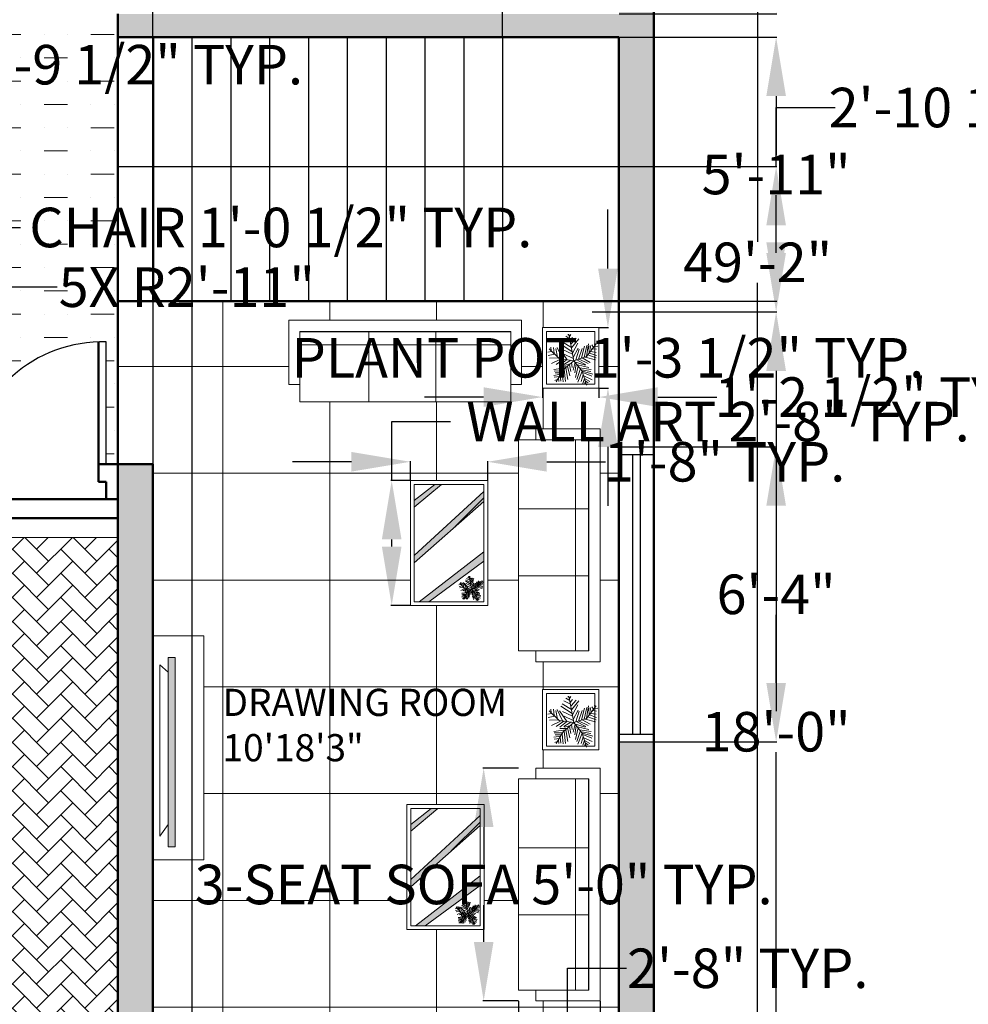
# Model space of a CAD drawing. Units: inches. Extents: x 26 to 14419, y 2 to 3479.
# Tile 3 of 9: x 13759 to 14003, y 2946 to 3199. Entities that reach past the tile are written whole.
import ezdxf

# ---------------------------------------------------------------- set-up
doc = ezdxf.new("R2010")
doc.units = ezdxf.units.IN
doc.header["$MEASUREMENT"] = 0
for name, color, linetype, lineweight in [('A-ANNO-DIMS', 2, 'Continuous', 18), ('A-AREA-IDEN', 7, 'Continuous', 18), ('A-DOOR', 4, 'Continuous', 25), ('A-FLOR-PATT', 252, 'Continuous', 13), ('A-FLOR-STRS', 2, 'Continuous', 25), ('A-FURN', 8, 'Continuous', 18), ('A-GLAZ', 3, 'Continuous', 25), ('A-WALL', 7, 'Continuous', 50), ('L-PLNT', 3, 'Continuous', 13)]:
    doc.layers.add(name, color=color, linetype=linetype, lineweight=lineweight)
doc.styles.get("Standard").update_dxf_attribs({"font": 'arial.ttf'})
doc.dimstyles.get("Standard").update_dxf_attribs({"dimtxt": 10.18, "dimasz": 15.18, "dimexe": 0.18, "dimexo": 0.0625, "dimgap": 0.09, "dimtad": 0, "dimtih": 1, "dimtoh": 1, "dimdec": 0, "dimzin": 0, "dimdsep": 46, "dimlunit": 3, "dimtxsty": 'Standard', "dimcen": 0.09, "dimadec": 0, "dimazin": 0, "dimtfac": 1, "dimtdec": 0, "dimtofl": 0, "dimtmove": 0, "dimatfit": 3, "dimfxl": 1, "dimtolj": 1, "dimtzin": 0, "dimarcsym": 0})

# ---------------------------------------------------------------- blocks, each defined once
blk = doc.blocks.new('*U5')
for p, q in [((-7.288, 39.707), (-21.778, 46.673)), ((-8.737, 47.138), (-17.069, 52.711)), ((-10.186, 53.64), (-13.084, 55.962)), ((0, 0), (-10.5, 57)), ((-9.099, 51.782), (-6.563, 55.962)), ((-7.65, 43.423), (-2.578, 49.46)), ((-5.839, 35.992), (4.667, 48.067)), ((-5.114, 27.632), (10.463, 46.673)), ((-31.5, 4.5), (-52.5, 25.5)), ((-48.585, 21.131), (-49.309, 29.026)), ((-43.513, 28.561), (-42.427, 15.558)), ((-38.442, 26.239), (-34.819, 7.663)), ((-35.544, 28.097), (-24.314, 3.947)), ((-14.533, 2.09), (-30.834, 25.31)), ((-3.665, 19.273), (-27.574, 35.527)), ((-5.114, 28.097), (-24.676, 40.636)), ((-24.314, 23.917), (-2.941, 13.7)), ((-2.941, 16.486), (8.652, 37.85)), ((-1.129, 6.734), (9.014, 26.704)), ((3.942, 1.625), (11.187, 24.381)), ((10.101, 3.483), (17.708, 26.239)), ((16.259, 5.805), (23.142, 31.348)), ((22.055, 7.198), (27.489, 32.277)), ((27, 9), (48, 36)), ((27.127, 9.056), (31.112, 35.992)), ((31.836, 30.883), (32.561, 16.486)), ((35.096, 32.741), (37.27, 22.524)), ((38.719, 34.134), (41.979, 28.561)), ((40.53, 25.775), (48.862, 24.846)), ((43.791, 29.954), (51.036, 30.883)), ((44.153, 36.456), (45.239, 32.741)), ((-47.498, 19.737), (-55.83, 18.344)), ((-40.615, 13.7), (-55.105, 10.913)), ((-33.37, 6.269), (-52.207, 5.34)), ((-28.299, 3.483), (-47.86, -5.805)), ((-21.416, 3.018), (-38.079, -8.128)), ((0, 0), (-31.5, 4.5)), ((-15.982, 2.09), (-30.11, -9.521)), ((0, 0), (-22.5, -19.5)), ((-6.563, 1.161), (-21.416, -8.128)), ((-20.691, 13.7), (-1.129, 4.876)), ((0, 0), (27, 9)), ((0, 0), (18, -22.5)), ((6.478, 1.625), (26.04, -8.592)), ((11.187, 3.483), (30.749, -5.805)), ((18.07, 5.805), (35.096, -3.483)), ((24.229, 7.663), (46.688, 1.625)), ((29.662, 12.307), (48.137, 6.269)), ((33.285, 16.486), (48.862, 10.913)), ((36.183, 19.737), (48.137, 17.88)), ((-17.431, -15.094), (-42.789, -18.809)), ((-22.5, -19.5), (-37.5, -45)), ((-15.257, -12.772), (-30.11, -12.772)), ((-20.691, -18.345), (-17.793, -44.352)), ((-6.563, -5.805), (-19.967, -9.985)), ((-17.069, -15.094), (-12.721, -40.172)), ((-13.446, -11.378), (-8.737, -32.741)), ((-9.461, -8.592), (-6.201, -23.453)), ((-4.752, -3.483), (-3.665, -14.629)), ((2.493, -3.019), (-1.491, -20.202)), ((1.769, -2.555), (24.229, -9.521)), ((5.029, -6.27), (2.131, -25.775)), ((9.014, -11.378), (3.58, -35.992)), ((14.085, -16.951), (6.478, -40.172)), ((7.565, -9.056), (32.198, -14.629)), ((12.274, -15.094), (36.907, -18.809)), ((16.259, -19.738), (36.183, -22.989)), ((-28.299, -29.026), (-42.789, -31.348)), ((-24.314, -21.596), (-42.427, -22.06)), ((-30.834, -34.135), (-42.427, -35.528)), ((-34.457, -39.708), (-40.978, -42.494)), ((-26.849, -26.24), (-40.253, -25.775)), ((-32.646, -36.921), (-31.921, -44.352)), ((-29.023, -30.884), (-27.936, -43.887)), ((-25.038, -23.918), (-22.865, -45.281)), ((18.07, -22.524), (8.289, -45.745)), ((20.244, -30.419), (15.897, -44.816)), ((18, -22.5), (27, -52.5)), ((18.433, -22.524), (40.53, -29.026)), ((19.157, -25.311), (38.719, -33.206)), ((22.78, -37.85), (19.519, -48.532)), ((21.331, -32.741), (39.081, -40.636)), ((22.78, -38.314), (34.372, -44.816)), ((24.591, -45.745), (23.142, -50.854)), ((24.591, -43.423), (30.749, -47.603)), ((26.764, -49.925), (28.213, -50.854))]:
    blk.add_line(p, q)
blk = doc.blocks.new('*D7')
at = {"layer": 'A-ANNO-DIMS', "color": 0, "lineweight": -2, "transparency": 16777216}
for p, q in [((13922.15, 3432), (13949, 3432)), ((13948.82, 3416.82), (13948.82, 3142.28)), ((13948.82, 2857.18), (13948.82, 3131.71)), ((13922.15, 2842), (13949, 2842))]:
    blk.add_line(p, q, dxfattribs=at)
at = {"layer": 'A-ANNO-DIMS', "color": 0, "transparency": 16777216}
for points in [[(13946.29, 3416.82), (13951.35, 3416.82), (13948.82, 3432)], [(13946.29, 2857.18), (13951.35, 2857.18), (13948.82, 2842)]]:
    blk.add_solid(points, dxfattribs=at)
at = {"layer": 'Defpoints', "color": 0, "transparency": 16777216}
for p in [(13922.09, 3432), (13922.09, 2842), (13948.82, 2842)]:
    blk.add_point(p, dxfattribs=at)
at = {"layer": 'A-ANNO-DIMS', "color": 0, "transparency": 16777216, "insert": (13948.82, 3137), "char_height": 10.18, "attachment_point": 5}
blk.add_mtext('\\A1;49\'-2"', dxfattribs=at)
blk = doc.blocks.new('SOFA-3SEAT')
for points in [[(2.79, 18.06), (2.79, 4.46), (0, 4.46), (0, 20.99), (2.79, 20.99)], [(2.79, 20.99), (59.95, 20.99)], [(57.16, 20.99), (59.95, 20.99), (59.95, 4.46), (57.16, 4.46), (57.16, 18.06)], [(57.16, 18.06), (2.79, 18.06)]]:
    blk.add_lwpolyline(points)
blk.add_lwpolyline([(2.79, 18.02), (57.16, 18.02), (57.16, 0), (2.79, 0)], close=True)
blk = doc.blocks.new('DOOR-DOUBLE')
for p, q in [((0, 0), (0, 31.5)), ((72, 0), (72, 31.5)), ((36.16, 0), (35.84, 0))]:
    blk.add_line(p, q)
for centre, start, end in [((1, -3.5), 5.7368, 91.6366), ((71, -3.5), 88.3634, 174.2632)]:
    blk.add_arc(centre, 35.01, start, end)
blk = doc.blocks.new('WALL-ART')
for p, q in [((6.28, 31.2), (1, 27.1)), ((8.01, 31.2), (1, 25.34)), ((18.91, 29.38), (1, 12.87)), ((18.91, 26.84), (1, 10.99)), ((18.91, 13.81), (2.23, 1)), ((18.91, 11.4), (4.72, 1))]:
    blk.add_line(p, q)
for points in [[(0, 32.2), (19.91, 32.2), (19.91, 0), (0, 0)], [(1, 31.2), (18.91, 31.2), (18.91, 1), (1, 1)]]:
    blk.add_lwpolyline(points, close=True)
blk = doc.blocks.new('PLANT-POT')
for points in [[(0, 15.58), (14.52, 15.58), (14.52, 0), (0, 0)], [(1, 14.58), (13.52, 14.58), (13.52, 1), (1, 1)]]:
    blk.add_lwpolyline(points, close=True)
blk = doc.blocks.new('*D23')
at = {"layer": 'A-ANNO-DIMS', "color": 0, "lineweight": -2, "transparency": 16777216}
for p, q in [((13716.08, 3147.8), (13716.08, 3145.8)), ((13728.65, 3147.8), (13728.65, 3145.8)), ((13700.9, 3145.98), (13685.72, 3145.98)), ((13743.83, 3145.98), (13759.01, 3145.98))]:
    blk.add_line(p, q, dxfattribs=at)
at = {"layer": 'A-ANNO-DIMS', "color": 0, "transparency": 16777216}
for points in [[(13700.9, 3148.51), (13700.9, 3143.45), (13716.08, 3145.98)], [(13743.83, 3148.51), (13743.83, 3143.45), (13728.65, 3145.98)]]:
    blk.add_solid(points, dxfattribs=at)
at = {"layer": 'Defpoints', "color": 0, "transparency": 16777216}
for p in [(13716.08, 3147.87), (13728.65, 3147.87), (13728.65, 3145.98)]:
    blk.add_point(p, dxfattribs=at)
at = {"layer": 'A-ANNO-DIMS', "color": 0, "transparency": 16777216, "insert": (13826.02, 3145.98), "char_height": 10.18, "attachment_point": 5}
blk.add_mtext('\\A1;CHAIR 1\'-0 1/2" TYP.', dxfattribs=at)
blk = doc.blocks.new('*D24')
at = {"layer": 'A-ANNO-DIMS', "color": 0, "lineweight": -2, "transparency": 16777216}
for p, q in [((13730.53, 3172.73), (13730.53, 3187.91)), ((13730.53, 3187.91), (13745.71, 3187.91)), ((13728.71, 3157.55), (13730.71, 3157.55)), ((13728.71, 3147.87), (13730.71, 3147.87)), ((13730.53, 3132.69), (13730.53, 3117.51))]:
    blk.add_line(p, q, dxfattribs=at)
at = {"layer": 'A-ANNO-DIMS', "color": 0, "transparency": 16777216}
for points in [[(13728, 3172.73), (13733.06, 3172.73), (13730.53, 3157.55)], [(13728, 3132.69), (13733.06, 3132.69), (13730.53, 3147.87)]]:
    blk.add_solid(points, dxfattribs=at)
at = {"layer": 'Defpoints', "color": 0, "transparency": 16777216}
for p in [(13728.65, 3157.55), (13730.53, 3157.55), (13728.65, 3147.87)]:
    blk.add_point(p, dxfattribs=at)
at = {"layer": 'A-ANNO-DIMS', "color": 0, "transparency": 16777216, "insert": (13788.69, 3187.91), "char_height": 10.18, "attachment_point": 5}
blk.add_mtext('\\A1;0\'-9 1/2" TYP.', dxfattribs=at)
blk = doc.blocks.new('*D30')
at = {"layer": 'A-ANNO-DIMS', "color": 0, "lineweight": -2, "transparency": 16777216}
for p, q in [((13899.89, 2940.02), (13899.89, 2955.2)), ((13899.89, 2955.2), (13915.07, 2955.2)), ((13889.15, 2940.02), (13900.07, 2940.02)), ((13899.89, 2923.18), (13899.89, 2924.84)), ((13889.15, 2908), (13900.07, 2908))]:
    blk.add_line(p, q, dxfattribs=at)
at = {"layer": 'A-ANNO-DIMS', "color": 0, "transparency": 16777216}
for points in [[(13897.36, 2924.84), (13902.42, 2924.84), (13899.89, 2940.02)], [(13897.36, 2923.18), (13902.42, 2923.18), (13899.89, 2908)]]:
    blk.add_solid(points, dxfattribs=at)
at = {"layer": 'Defpoints', "color": 0, "transparency": 16777216}
for p in [(13889.09, 2940.02), (13899.89, 2940.02), (13889.09, 2908)]:
    blk.add_point(p, dxfattribs=at)
at = {"layer": 'A-ANNO-DIMS', "color": 0, "transparency": 16777216, "insert": (13946.27, 2955.2), "char_height": 10.18, "attachment_point": 5}
blk.add_mtext('\\A1;2\'-8" TYP.', dxfattribs=at)
blk = doc.blocks.new('*D31')
at = {"layer": 'A-ANNO-DIMS', "color": 0, "lineweight": -2, "transparency": 16777216}
for p, q in [((13887.2, 3006.75), (13878.09, 3006.75)), ((13878.27, 2991.57), (13878.27, 2982.14)), ((13878.27, 2961.99), (13878.27, 2971.42)), ((13887.2, 2946.81), (13878.09, 2946.81))]:
    blk.add_line(p, q, dxfattribs=at)
at = {"layer": 'A-ANNO-DIMS', "color": 0, "transparency": 16777216}
for points in [[(13875.74, 2991.57), (13880.8, 2991.57), (13878.27, 3006.75)], [(13875.74, 2961.99), (13880.8, 2961.99), (13878.27, 2946.81)]]:
    blk.add_solid(points, dxfattribs=at)
at = {"layer": 'Defpoints', "color": 0, "transparency": 16777216}
for p in [(13887.26, 3006.75), (13878.27, 2946.81), (13887.26, 2946.81)]:
    blk.add_point(p, dxfattribs=at)
at = {"layer": 'A-ANNO-DIMS', "color": 0, "transparency": 16777216, "insert": (13878.27, 2976.78), "char_height": 10.18, "attachment_point": 5}
blk.add_mtext('\\A1;3-SEAT SOFA 5\'-0" TYP.', dxfattribs=at)
blk = doc.blocks.new('*D32')
at = {"layer": 'A-ANNO-DIMS', "color": 0, "lineweight": -2, "transparency": 16777216}
for p, q in [((13887.26, 2946.75), (13887.26, 2937.64)), ((13908.25, 2946.75), (13908.25, 2937.64)), ((13872.08, 2937.82), (13856.9, 2937.82)), ((13923.43, 2937.82), (13938.61, 2937.82))]:
    blk.add_line(p, q, dxfattribs=at)
at = {"layer": 'A-ANNO-DIMS', "color": 0, "transparency": 16777216}
for points in [[(13872.08, 2940.35), (13872.08, 2935.29), (13887.26, 2937.82)], [(13923.43, 2940.35), (13923.43, 2935.29), (13908.25, 2937.82)]]:
    blk.add_solid(points, dxfattribs=at)
at = {"layer": 'Defpoints', "color": 0, "transparency": 16777216}
for p in [(13887.26, 2946.81), (13908.25, 2946.81), (13908.25, 2937.82)]:
    blk.add_point(p, dxfattribs=at)
at = {"layer": 'A-ANNO-DIMS', "color": 0, "transparency": 16777216, "insert": (13969.25, 2937.82), "char_height": 10.18, "attachment_point": 5}
blk.add_mtext('\\A1;1\'-9" TYP.', dxfattribs=at)
blk = doc.blocks.new('*D41')
at = {"layer": 'A-ANNO-DIMS', "color": 0, "lineweight": -2, "transparency": 16777216}
for p, q in [((13854.58, 3080.81), (13854.58, 3095.99)), ((13854.58, 3095.99), (13869.76, 3095.99)), ((13859.35, 3080.81), (13854.4, 3080.81)), ((13854.58, 3063.79), (13854.58, 3065.63)), ((13859.35, 3048.61), (13854.4, 3048.61))]:
    blk.add_line(p, q, dxfattribs=at)
at = {"layer": 'A-ANNO-DIMS', "color": 0, "transparency": 16777216}
for points in [[(13852.05, 3065.63), (13857.11, 3065.63), (13854.58, 3080.81)], [(13852.05, 3063.79), (13857.11, 3063.79), (13854.58, 3048.61)]]:
    blk.add_solid(points, dxfattribs=at)
at = {"layer": 'Defpoints', "color": 0, "transparency": 16777216}
for p in [(13854.58, 3080.81), (13859.41, 3080.81), (13859.41, 3048.61)]:
    blk.add_point(p, dxfattribs=at)
at = {"layer": 'A-ANNO-DIMS', "color": 0, "transparency": 16777216, "insert": (13938.62, 3095.99), "char_height": 10.18, "attachment_point": 5}
blk.add_mtext('\\A1;WALL ART 2\'-8" TYP.', dxfattribs=at)
blk = doc.blocks.new('*D42')
at = {"layer": 'A-ANNO-DIMS', "color": 0, "lineweight": -2, "transparency": 16777216}
for p, q in [((13844.23, 3085.64), (13829.05, 3085.64)), ((13859.41, 3080.87), (13859.41, 3085.82)), ((13879.32, 3080.87), (13879.32, 3085.82)), ((13894.5, 3085.64), (13909.68, 3085.64))]:
    blk.add_line(p, q, dxfattribs=at)
at = {"layer": 'A-ANNO-DIMS', "color": 0, "transparency": 16777216}
for points in [[(13844.23, 3088.17), (13844.23, 3083.11), (13859.41, 3085.64)], [(13894.5, 3088.17), (13894.5, 3083.11), (13879.32, 3085.64)]]:
    blk.add_solid(points, dxfattribs=at)
at = {"layer": 'Defpoints', "color": 0, "transparency": 16777216}
for p in [(13879.32, 3085.64), (13859.41, 3080.81), (13879.32, 3080.81)]:
    blk.add_point(p, dxfattribs=at)
at = {"layer": 'A-ANNO-DIMS', "color": 0, "transparency": 16777216, "insert": (13940.31, 3085.64), "char_height": 10.18, "attachment_point": 5}
blk.add_mtext('\\A1;1\'-8" TYP.', dxfattribs=at)
blk = doc.blocks.new('*D45')
at = {"layer": 'A-ANNO-DIMS', "color": 0, "lineweight": -2, "transparency": 16777216}
for p, q in [((13910.27, 3135.39), (13910.27, 3150.57)), ((13907.99, 3120.21), (13910.45, 3120.21)), ((13907.99, 3104.63), (13910.45, 3104.63)), ((13910.27, 3089.45), (13910.27, 3074.27))]:
    blk.add_line(p, q, dxfattribs=at)
at = {"layer": 'A-ANNO-DIMS', "color": 0, "transparency": 16777216}
for points in [[(13907.74, 3135.39), (13912.8, 3135.39), (13910.27, 3120.21)], [(13907.74, 3089.45), (13912.8, 3089.45), (13910.27, 3104.63)]]:
    blk.add_solid(points, dxfattribs=at)
at = {"layer": 'Defpoints', "color": 0, "transparency": 16777216}
for p in [(13907.93, 3120.21), (13910.27, 3120.21), (13907.93, 3104.63)]:
    blk.add_point(p, dxfattribs=at)
at = {"layer": 'A-ANNO-DIMS', "color": 0, "transparency": 16777216, "insert": (13910.27, 3112.42), "char_height": 10.18, "attachment_point": 5}
blk.add_mtext('\\A1;PLANT POT 1\'-3 1/2" TYP.', dxfattribs=at)
blk = doc.blocks.new('*D46')
at = {"layer": 'A-ANNO-DIMS', "color": 0, "lineweight": -2, "transparency": 16777216}
for p, q in [((13893.41, 3104.57), (13893.41, 3102.12)), ((13907.93, 3104.57), (13907.93, 3102.12)), ((13878.23, 3102.3), (13863.05, 3102.3)), ((13923.11, 3102.3), (13938.29, 3102.3))]:
    blk.add_line(p, q, dxfattribs=at)
at = {"layer": 'A-ANNO-DIMS', "color": 0, "transparency": 16777216}
for points in [[(13878.23, 3104.83), (13878.23, 3099.77), (13893.41, 3102.3)], [(13923.11, 3104.83), (13923.11, 3099.77), (13907.93, 3102.3)]]:
    blk.add_solid(points, dxfattribs=at)
at = {"layer": 'Defpoints', "color": 0, "transparency": 16777216}
for p in [(13893.41, 3104.63), (13907.93, 3104.63), (13907.93, 3102.3)]:
    blk.add_point(p, dxfattribs=at)
at = {"layer": 'A-ANNO-DIMS', "color": 0, "transparency": 16777216, "insert": (13980.79, 3102.3), "char_height": 10.18, "attachment_point": 5}
blk.add_mtext('\\A1;1\'-2 1/2" TYP.', dxfattribs=at)
blk = doc.blocks.new('*D66')
at = {"layer": 'A-ANNO-DIMS', "color": 0, "lineweight": -2, "transparency": 16777216}
for p, q in [((13906.22, 3124.24), (13953.77, 3124.24)), ((13953.59, 3109.06), (13953.59, 3021.41)), ((13953.59, 2923.18), (13953.59, 3010.83)), ((13913.15, 2908), (13953.77, 2908))]:
    blk.add_line(p, q, dxfattribs=at)
at = {"layer": 'A-ANNO-DIMS', "color": 0, "transparency": 16777216}
for points in [[(13951.06, 3109.06), (13956.12, 3109.06), (13953.59, 3124.24)], [(13951.06, 2923.18), (13956.12, 2923.18), (13953.59, 2908)]]:
    blk.add_solid(points, dxfattribs=at)
at = {"layer": 'Defpoints', "color": 0, "transparency": 16777216}
for p in [(13906.16, 3124.24), (13953.59, 3124.24), (13913.09, 2908)]:
    blk.add_point(p, dxfattribs=at)
at = {"layer": 'A-ANNO-DIMS', "color": 0, "transparency": 16777216, "insert": (13953.59, 3016.12), "char_height": 10.18, "attachment_point": 5}
blk.add_mtext('\\A1;18\'-0"', dxfattribs=at)
blk = doc.blocks.new('*D67')
at = {"layer": 'A-ANNO-DIMS', "color": 0, "lineweight": -2, "transparency": 16777216}
for p, q in [((13913.15, 3195), (13953.77, 3195)), ((13953.59, 3179.82), (13953.59, 3164.91)), ((13953.59, 3139.42), (13953.59, 3154.33)), ((13906.22, 3124.24), (13953.77, 3124.24))]:
    blk.add_line(p, q, dxfattribs=at)
at = {"layer": 'A-ANNO-DIMS', "color": 0, "transparency": 16777216}
for points in [[(13951.06, 3179.82), (13956.12, 3179.82), (13953.59, 3195)], [(13951.06, 3139.42), (13956.12, 3139.42), (13953.59, 3124.24)]]:
    blk.add_solid(points, dxfattribs=at)
at = {"layer": 'Defpoints', "color": 0, "transparency": 16777216}
for p in [(13913.09, 3195), (13953.59, 3195), (13906.16, 3124.24)]:
    blk.add_point(p, dxfattribs=at)
at = {"layer": 'A-ANNO-DIMS', "color": 0, "transparency": 16777216, "insert": (13953.59, 3159.62), "char_height": 10.18, "attachment_point": 5}
blk.add_mtext('\\A1;5\'-11"', dxfattribs=at)
blk = doc.blocks.new('*D68')
at = {"layer": 'A-ANNO-DIMS', "color": 0, "lineweight": -2, "transparency": 16777216}
for p, q in [((13953.59, 3216.18), (13953.59, 3231.36)), ((13953.59, 3231.36), (13968.77, 3231.36)), ((13913.15, 3201), (13953.77, 3201)), ((13913.15, 3195), (13953.77, 3195)), ((13953.59, 3179.82), (13953.59, 3164.64))]:
    blk.add_line(p, q, dxfattribs=at)
at = {"layer": 'A-ANNO-DIMS', "color": 0, "transparency": 16777216}
for points in [[(13951.06, 3216.18), (13956.12, 3216.18), (13953.59, 3201)], [(13951.06, 3179.82), (13956.12, 3179.82), (13953.59, 3195)]]:
    blk.add_solid(points, dxfattribs=at)
at = {"layer": 'Defpoints', "color": 0, "transparency": 16777216}
for p in [(13913.09, 3201), (13953.59, 3201), (13913.09, 3195)]:
    blk.add_point(p, dxfattribs=at)
at = {"layer": 'A-ANNO-DIMS', "color": 0, "transparency": 16777216, "insert": (13982.39, 3231.36), "char_height": 10.18, "attachment_point": 5}
blk.add_mtext('\\A1;0\'-6"', dxfattribs=at)
blk = doc.blocks.new('*D72')
at = {"layer": 'A-ANNO-DIMS', "color": 0, "lineweight": -2, "transparency": 16777216}
for p, q in [((13922.15, 3089.5), (13953.77, 3089.5)), ((13953.59, 3074.32), (13953.59, 3056.78)), ((13953.59, 3028.68), (13953.59, 3046.21)), ((13922.15, 3013.5), (13953.77, 3013.5))]:
    blk.add_line(p, q, dxfattribs=at)
at = {"layer": 'A-ANNO-DIMS', "color": 0, "transparency": 16777216}
for points in [[(13951.06, 3074.32), (13956.12, 3074.32), (13953.59, 3089.5)], [(13951.06, 3028.68), (13956.12, 3028.68), (13953.59, 3013.5)]]:
    blk.add_solid(points, dxfattribs=at)
at = {"layer": 'Defpoints', "color": 0, "transparency": 16777216}
for p in [(13922.09, 3089.5), (13953.59, 3089.5), (13922.09, 3013.5)]:
    blk.add_point(p, dxfattribs=at)
at = {"layer": 'A-ANNO-DIMS', "color": 0, "transparency": 16777216, "insert": (13953.59, 3051.5), "char_height": 10.18, "attachment_point": 5}
blk.add_mtext('\\A1;6\'-4"', dxfattribs=at)
blk = doc.blocks.new('*D81')
at = {"layer": 'A-ANNO-DIMS', "color": 0, "lineweight": -2, "transparency": 16777216}
for p, q in [((13793.09, 3195.06), (13793.09, 3463.68)), ((13808.27, 3463.5), (13824.54, 3463.5)), ((13867.96, 3463.5), (13851.69, 3463.5)), ((13883.14, 3195.06), (13883.14, 3463.68))]:
    blk.add_line(p, q, dxfattribs=at)
at = {"layer": 'A-ANNO-DIMS', "color": 0, "transparency": 16777216}
for points in [[(13808.27, 3466.03), (13808.27, 3460.97), (13793.09, 3463.5)], [(13867.96, 3466.03), (13867.96, 3460.97), (13883.14, 3463.5)]]:
    blk.add_solid(points, dxfattribs=at)
at = {"layer": 'Defpoints', "color": 0, "transparency": 16777216}
for p in [(13883.14, 3463.5), (13793.09, 3195), (13883.14, 3195)]:
    blk.add_point(p, dxfattribs=at)
at = {"layer": 'A-ANNO-DIMS', "color": 0, "transparency": 16777216, "insert": (13838.12, 3463.5), "char_height": 10.18, "attachment_point": 5}
blk.add_mtext('\\A1;7\'-6"', dxfattribs=at)
blk = doc.blocks.new('*D82')
at = {"layer": 'A-ANNO-DIMS', "color": 0, "lineweight": -2, "transparency": 16777216}
for p, q in [((13793.09, 3126.93), (13793.09, 2810.32)), ((13803.14, 3126.93), (13803.14, 2810.32)), ((13777.91, 2810.5), (13762.73, 2810.5)), ((13818.32, 2810.5), (13833.5, 2810.5))]:
    blk.add_line(p, q, dxfattribs=at)
at = {"layer": 'A-ANNO-DIMS', "color": 0, "transparency": 16777216}
for points in [[(13777.91, 2813.03), (13777.91, 2807.97), (13793.09, 2810.5)], [(13818.32, 2813.03), (13818.32, 2807.97), (13803.14, 2810.5)]]:
    blk.add_solid(points, dxfattribs=at)
at = {"layer": 'Defpoints', "color": 0, "transparency": 16777216}
for p in [(13793.09, 3127), (13803.14, 3127), (13803.14, 2810.5)]:
    blk.add_point(p, dxfattribs=at)
at = {"layer": 'A-ANNO-DIMS', "color": 0, "transparency": 16777216, "insert": (13851.07, 2810.5), "char_height": 10.18, "attachment_point": 5}
blk.add_mtext('\\A1;0\'-10"', dxfattribs=at)
blk = doc.blocks.new('*D83')
at = {"layer": 'A-ANNO-DIMS', "color": 0, "lineweight": -2, "transparency": 16777216}
for p, q in [((13953.59, 3161.69), (13953.59, 3176.87)), ((13953.59, 3176.87), (13968.77, 3176.87)), ((13883.2, 3161.69), (13953.77, 3161.69)), ((13953.59, 3142.18), (13953.59, 3146.51)), ((13883.2, 3127), (13953.77, 3127))]:
    blk.add_line(p, q, dxfattribs=at)
at = {"layer": 'A-ANNO-DIMS', "color": 0, "transparency": 16777216}
for points in [[(13951.06, 3146.51), (13956.12, 3146.51), (13953.59, 3161.69)], [(13951.06, 3142.18), (13956.12, 3142.18), (13953.59, 3127)]]:
    blk.add_solid(points, dxfattribs=at)
at = {"layer": 'Defpoints', "color": 0, "transparency": 16777216}
for p in [(13883.14, 3161.69), (13953.59, 3161.69), (13883.14, 3127)]:
    blk.add_point(p, dxfattribs=at)
at = {"layer": 'A-ANNO-DIMS', "color": 0, "transparency": 16777216, "insert": (13998.29, 3176.87), "char_height": 10.18, "attachment_point": 5}
blk.add_mtext('\\A1;2\'-10 1/2"', dxfattribs=at)
blk = doc.blocks.new('*D121')
at = {"layer": 'A-ANNO-DIMS', "color": 0, "lineweight": -2, "transparency": 16777216}
for p, q in [((13753.25, 3130.6), (13743.23, 3119.2)), ((13768.43, 3130.6), (13753.25, 3130.6)), ((13710, 3081.5), (13710.18, 3081.5)), ((13710.09, 3081.41), (13710.09, 3081.59))]:
    blk.add_line(p, q, dxfattribs=at)
at = {"layer": 'A-ANNO-DIMS', "color": 0, "transparency": 16777216}
blk.add_solid([(13741.33, 3120.87), (13745.13, 3117.53), (13733.21, 3107.8)], dxfattribs=at)
at = {"layer": 'Defpoints', "color": 0, "transparency": 16777216}
for p in [(13733.21, 3107.8), (13710.09, 3081.5)]:
    blk.add_point(p, dxfattribs=at)
at = {"layer": 'A-ANNO-DIMS', "color": 0, "transparency": 16777216, "insert": (13801.81, 3130.6), "char_height": 10.18, "attachment_point": 5}
blk.add_mtext('\\A1;5X R2\'-11"', dxfattribs=at)

msp = doc.modelspace()

# ---------------------------------------------------------------- hatches: boundary and pattern name
at = {"layer": 'A-FLOR-PATT'}
h = msp.add_hatch(color=256, dxfattribs=at)
h.dxf.hatch_style = 1
h.paths.add_polyline_path([(13922.09, 3432), (13659.09, 3432), (13659.09, 2842), (13668.09, 2842), (13668.09, 2851), (13668.09, 2899), (13668.09, 2908), (13668.09, 3076), (13706.09, 3076), (13706.09, 3085), (13668.09, 3085), (13668.09, 3249), (13712.76, 3249), (13712.76, 3255), (13668.09, 3255), (13668.09, 3375), (13720.94, 3375), (13720.94, 3378, -0.017236), (13720.94, 3380), (13720.94, 3381), (13668.09, 3381), (13668.09, 3423), (13784.09, 3423), (13784.09, 3381), (13753.94, 3381), (13753.94, 3375), (13784.09, 3375), (13784.09, 3255), (13758.77, 3255), (13758.77, 3249), (13784.09, 3249), (13793.09, 3249), (13793.09, 3255), (13793.09, 3423), (13913.09, 3423), (13913.09, 3255), (13832.09, 3255), (13832.09, 3254, -0.014283), (13832.09, 3252), (13832.09, 3249), (13836.57, 3249), (13836.57, 3234), (13839.57, 3234, -0.017236), (13841.57, 3234), (13842.57, 3234), (13842.57, 3249), (13913.09, 3249), (13913.09, 3201), (13892.46, 3201), (13793.09, 3201), (13784.09, 3201), (13784.09, 3195), (13793.09, 3195), (13913.09, 3195), (13913.09, 3127), (13922.09, 3127)])
h.paths.add_polyline_path([(13922.09, 3013.5), (13913.09, 3013.5), (13913.09, 2908), (13892.09, 2908), (13892.09, 2899), (13913.09, 2899), (13913.09, 2851), (13793.09, 2851), (13784.09, 2851), (13784.09, 2842), (13922.09, 2842)], flags=17)
h.paths.add_polyline_path([(13793.09, 3085), (13784.09, 3085), (13784.09, 3076), (13784.09, 3071.08), (13784.09, 3066.17), (13784.09, 2908), (13784.09, 2899.07), (13793.09, 2899), (13802.09, 2899), (13814.09, 2899), (13814.09, 2908), (13793.09, 2908)], flags=17)
h.paths.add_polyline_path([(14342.64, 3401.72), (14242.78, 3401.72), (14242.78, 3392.72), (14257.64, 3392.72), (14257.64, 3351.75), (14257.64, 3345.75), (14257.64, 3330.73), (14263.64, 3330.73), (14263.64, 3392.72), (14333.64, 3392.72), (14333.64, 3284.72), (14302.92, 3284.72), (14302.92, 3281.72, -0.022645), (14302.92, 3279.12), (14302.92, 3278.72), (14333.64, 3278.72), (14333.64, 3170.72), (14316.1, 3170.72), (14263.64, 3170.72), (14263.64, 3278.72), (14269.92, 3278.72), (14269.92, 3284.72), (14263.64, 3284.72), (14257.64, 3284.72), (14257.64, 3225.75), (14257.64, 3219.75), (14257.64, 3164.72), (14333.64, 3164.72), (14333.64, 3110.37), (14210.01, 3110.37), (14210.01, 3104.37), (14257.64, 3104.37), (14257.64, 3024), (14263.64, 3024), (14263.64, 3039.72), (14263.64, 3104.37), (14333.64, 3104.37), (14333.64, 3045.72), (14333.64, 3039.72), (14333.64, 2967.72), (14296.64, 2967.72), (14296.64, 2964.72, -0.017236), (14296.64, 2962.72), (14296.64, 2961.72), (14333.64, 2961.72), (14333.64, 2882.72), (14312.64, 2882.72), (14312.64, 2873.72), (14333.64, 2873.72), (14333.64, 2820.72), (14333.64, 2811.72), (14342.64, 2811.72)])
h.paths.add_polyline_path([(14088.64, 3219.75), (14218.64, 3219.75), (14218.64, 3222.75, -0.014283), (14218.64, 3224.75), (14218.64, 3225.75), (14088.64, 3225.75), (14088.64, 3345.75), (14088.64, 3351.75), (14088.64, 3392.72), (14193.93, 3392.72), (14193.93, 3351.75), (14140.64, 3351.75), (14140.64, 3345.75), (14170.7, 3345.75), (14218.64, 3345.75), (14218.64, 3348.75, -0.014283), (14218.64, 3350.75), (14218.64, 3351.75), (14199.93, 3351.75), (14199.93, 3392.72), (14214.78, 3392.72), (14214.78, 3401.72), (14079.64, 3401.72), (14079.64, 2811.72), (14088.64, 2811.72), (14088.64, 2820.72), (14088.64, 2873.72), (14116.21, 2873.72), (14116.21, 2876.57), (14116.21, 2882.72), (14088.64, 2882.72), (14088.64, 3039.72), (14216.01, 3039.72), (14216.01, 3065.37), (14215.01, 3065.37, -0.014283), (14213.01, 3065.37), (14210.01, 3065.37), (14210.01, 3045.72), (14154.64, 3045.72), (14148.64, 3045.72), (14088.64, 3045.72)])
h.paths.add_polyline_path([(14284.64, 2882.72), (14263.64, 2882.72), (14263.64, 2961.72), (14263.64, 2967.72), (14257.64, 2967.72), (14257.64, 2956.69), (14257.64, 2916.18), (14257.64, 2882.72), (14249.61, 2882.72), (14249.61, 2873.72), (14284.64, 2873.72)], flags=17)
h.paths.add_polyline_path([(14202.78, 2882.72), (14189.55, 2882.72), (14189.55, 2879.95), (14189.55, 2873.72), (14202.78, 2873.72)], flags=17)
h = msp.add_hatch(dxfattribs=at)
h.set_pattern_fill('MUDST', color=256, scale=24)
h.set_pattern_definition([(0, (61.093, 57.669), (12, 6), [6, -6, 0, -6, 0, -6])])
h.paths.add_polyline_path([(13756.28, 3375), (13750.94, 3375), (13720.94, 3375), (13706.54, 3375), (13706.54, 3255), (13712.76, 3255), (13712.76, 3249), (13668.09, 3249), (13668.09, 3085), (13709.09, 3085), (13709.09, 3116.5, -0.393405), (13744.93, 3085), (13745.25, 3085, -0.393405), (13781.09, 3116.5), (13781.09, 3085), (13784.09, 3085), (13784.09, 3127), (13784.09, 3195), (13784.09, 3201), (13793.09, 3201), (13836.57, 3201), (13836.57, 3204), (13836.57, 3234), (13836.57, 3249), (13832.09, 3249), (13832.09, 3254, 0.397579), (13798.09, 3288), (13798.09, 3252), (13796.09, 3252), (13796.09, 3249), (13793.09, 3249), (13784.09, 3249), (13758.77, 3249), (13758.77, 3255), (13784.09, 3255), (13784.09, 3303.43), (13756.28, 3303.43)])
h.paths.add_polyline_path([(13757.29, 3298.63), (13757.76, 3298.12), (13779.63, 3298.12), (13779.63, 3268.87), (13757.77, 3268.87), (13756.19, 3268.87), (13756.19, 3285.02), (13757.77, 3285.02), (13757.77, 3298.11), (13749.96, 3290.89), (13749.48, 3291.4)], flags=16)
h.paths.add_polyline_path([(13758.77, 3297.12), (13778.63, 3297.12), (13778.63, 3269.87), (13758.77, 3269.87)], flags=0)
h.paths.add_polyline_path([(13716.08, 3198.11), (13716.08, 3190.37), (13728.65, 3190.37), (13728.65, 3180.68), (13716.08, 3180.68), (13716.08, 3174.63), (13728.65, 3174.63), (13728.65, 3164.95), (13716.08, 3164.95), (13716.08, 3157.55), (13728.65, 3157.55), (13728.65, 3147.87), (13716.08, 3147.87), (13716.08, 3142.39), (13687.89, 3142.39), (13687.89, 3145.78), (13675.33, 3145.78), (13675.33, 3155.46), (13687.89, 3155.46), (13687.89, 3163.27), (13675.33, 3163.27), (13675.33, 3172.95), (13687.89, 3172.95), (13687.89, 3179.58), (13675.33, 3179.58), (13675.33, 3189.26), (13687.89, 3189.26), (13687.89, 3198.11)], flags=16)
h.paths.add_polyline_path([(13715.08, 3197.11), (13715.08, 3143.39), (13688.89, 3143.39), (13688.89, 3197.11)], flags=0)
h = msp.add_hatch(dxfattribs=at)
h.set_pattern_fill('NET', color=256, scale=220)
h.set_pattern_definition([(0, (61.093, 57.67), (0, 27.5), []), (90, (61.093, 57.67), (-27.5, 2e-15), [])])
h.paths.add_polyline_path([(13913.09, 3127), (13819.09, 3127), (13793.09, 3127), (13784.09, 3127), (13784.09, 3085), (13793.09, 3085), (13793.09, 3040.8), (13806.22, 3040.8), (13806.22, 2983.17), (13793.09, 2983.17), (13793.09, 2908), (13817.09, 2908), (13817.09, 2939.5, -0.393405), (13852.93, 2908), (13853.25, 2908, -0.393405), (13889.09, 2939.5), (13889.09, 2908), (13913.09, 2908)])
h.paths.add_polyline_path([(13878.38, 2997.35), (13878.38, 2965.16), (13858.47, 2965.16), (13858.47, 2997.35)], flags=16)
h.paths.add_polyline_path([(13859.47, 2996.35), (13877.38, 2996.35), (13877.38, 2966.16), (13859.47, 2966.16)], flags=0)
h.paths.add_polyline_path([(13859.41, 3048.61), (13859.41, 3080.81), (13879.32, 3080.81), (13879.32, 3048.61)], flags=16)
h.paths.add_polyline_path([(13860.41, 3049.61), (13860.41, 3079.81), (13878.32, 3079.81), (13878.32, 3049.61)], flags=0)
h.paths.add_polyline_path([(13887.26, 3003.97), (13891.72, 3003.97), (13891.72, 3006.75), (13908.25, 3006.75), (13908.25, 3003.97), (13908.25, 2946.81), (13891.72, 2946.81), (13887.26, 2949.6)], flags=16)
h.paths.add_polyline_path([(13887.26, 3036.93), (13887.26, 3091.3), (13891.72, 3091.3), (13891.72, 3094.09), (13908.25, 3094.09), (13908.25, 3091.3), (13908.25, 3034.14), (13891.72, 3034.14)], flags=16)
h.paths.add_polyline_path([(13893.41, 3027), (13907.93, 3027), (13907.93, 3011.42), (13893.41, 3011.42)], flags=16)
h.paths.add_polyline_path([(13874.64, 3054.21), (13874.87, 3054.49), (13874.86, 3054.52), (13872.61, 3055.96), (13872.7, 3055.53)], flags=0)
h.paths.add_polyline_path([(13873.75, 3054.27), (13874.59, 3055.26), (13872.48, 3056.28), (13872.52, 3055.73), (13872.77, 3055.19), (13873.25, 3054.5)], flags=0)
h.paths.add_polyline_path([(13873.61, 3052.85), (13873.55, 3052.9), (13873.56, 3052.82)], flags=0)
h.paths.add_polyline_path([(13872.76, 3051.79), (13871.09, 3051.54), (13872.51, 3051.58)], flags=0)
h.paths.add_polyline_path([(13894.41, 3026), (13906.93, 3026), (13906.93, 3012.42), (13894.41, 3012.42)], flags=0)
h.paths.add_polyline_path([(13905.32, 2986.18), (13905.32, 3003.97), (13901.96, 3003.97), (13901.96, 2986.18)], flags=0)
h.paths.add_polyline_path([(13901.96, 3073.51), (13905.32, 3073.51), (13905.32, 3091.3), (13901.96, 3091.3)], flags=0)
h.paths.add_polyline_path([(13874.39, 2970.25), (13874.4, 2970.28), (13874.29, 2970.36), (13874.25, 2970.32)], flags=0)
h.paths.add_polyline_path([(13830.89, 3101.09), (13830.89, 3105.55), (13828.1, 3105.55), (13828.1, 3122.08), (13830.89, 3122.08), (13888.05, 3122.08), (13888.05, 3105.55), (13885.26, 3101.09)], flags=16)
h.paths.add_polyline_path([(13848.68, 3115.79), (13848.68, 3119.15), (13830.89, 3119.15), (13830.89, 3115.79)], flags=0)
h.paths.add_polyline_path([(13893.41, 3104.63), (13893.41, 3120.21), (13907.93, 3120.21), (13907.93, 3104.63)], flags=16)
h.paths.add_polyline_path([(13894.41, 3105.63), (13894.41, 3119.21), (13906.93, 3119.21), (13906.93, 3105.63)], flags=0)
h = msp.add_hatch(dxfattribs=at)
h.set_pattern_fill('ANSI32', color=256, scale=8.9)
h.set_pattern_definition([(45, (74.4894, 52.822), (-2.3599689, 2.3599689), []), (45, (76.0627, 52.822), (-2.3599689, 2.3599689), [])])
h.paths.add_polyline_path([(13867.42, 3079.81), (13865.69, 3079.81), (13860.41, 3075.71), (13860.41, 3073.95)])
h.paths.add_polyline_path([(13878.32, 3075.46), (13878.32, 3077.99), (13860.41, 3061.49), (13860.41, 3059.6)])
h = msp.add_hatch(color=256, dxfattribs=at)
h.dxf.hatch_style = 1
h.paths.add_polyline_path([(13860.41, 3075.71), (13860.41, 3073.95), (13867.42, 3079.81), (13865.69, 3079.81)])
h.paths.add_polyline_path([(13878.32, 3075.46), (13878.32, 3077.99), (13860.41, 3061.49), (13860.41, 3059.6)])
h.paths.add_polyline_path([(13878.32, 3060.01), (13878.32, 3062.42), (13861.64, 3049.61), (13864.13, 3049.61)])
h = msp.add_hatch(dxfattribs=at)
h.set_pattern_fill('AR-HBONE', color=256, scale=1.1)
h.set_pattern_definition([(45, (61.093, 57.669), (0, 6.2225397), [13.2, -4.4]), (135, (64.2045, 60.7802), (5e-16, 6.2225397), [13.2, -4.4])])
h.paths.add_polyline_path([(13668.09, 2908), (13668.09, 2899), (13668.09, 2851), (13668.09, 2842), (13784.09, 2842), (13784.09, 2851), (13784.09, 2899), (13784.09, 2908), (13784.09, 3066.17), (13709.09, 3066.17), (13709.09, 3071.08), (13709.09, 3076), (13668.09, 3076)])
h = msp.add_hatch(color=256, dxfattribs=at)
h.dxf.hatch_style = 1
h.paths.add_polyline_path([(13798.84, 3035.21), (13797.05, 3035.21), (13797.05, 2986.49), (13798.84, 2986.49)])
h = msp.add_hatch(dxfattribs=at)
h.set_pattern_fill('ANSI32', color=256, scale=8.9)
h.set_pattern_definition([(45, (73.556, -30.634), (-2.3599689, 2.3599689), []), (45, (75.1292, -30.634), (-2.3599689, 2.3599689), [])])
h.paths.add_polyline_path([(13866.49, 2996.35), (13864.75, 2996.35), (13859.47, 2992.26), (13859.47, 2990.49)])
h.paths.add_polyline_path([(13877.38, 2992), (13877.38, 2994.53), (13859.47, 2978.03), (13859.47, 2976.14)])
h = msp.add_hatch(color=256, dxfattribs=at)
h.dxf.hatch_style = 1
h.paths.add_polyline_path([(13866.49, 2996.35), (13864.75, 2996.35), (13859.47, 2992.26), (13859.47, 2990.49)])
h.paths.add_polyline_path([(13877.38, 2992), (13877.38, 2994.53), (13859.47, 2978.03), (13859.47, 2976.14)])
h.paths.add_polyline_path([(13877.38, 2976.55), (13877.38, 2978.96), (13860.71, 2966.16), (13863.19, 2966.16)])

# ---------------------------------------------------------------- linework, layer by layer
at = {"layer": 'A-FLOR-STRS'}
for p, q in [((13803.14, 3195), (13803.14, 3127)), ((13813.14, 3195), (13813.14, 3127)), ((13823.14, 3195), (13823.14, 3127)), ((13833.14, 3195), (13833.14, 3127)), ((13843.14, 3195), (13843.14, 3127)), ((13853.14, 3195), (13853.14, 3127)), ((13863.14, 3195), (13863.14, 3127)), ((13873.14, 3195), (13873.14, 3127)), ((13883.14, 3195), (13883.14, 3127)), ((13784.09, 3161.69), (13883.14, 3161.69))]:
    msp.add_line(p, q, dxfattribs=at)
at = {"layer": 'A-FURN'}
for p, q in [((13848.68, 3119.11), (13848.68, 3101.09)), ((13865.91, 3119.11), (13865.91, 3101.09)), ((13830.89, 3115.79), (13885.26, 3115.79)), ((13901.96, 3091.3), (13901.96, 3036.93)), ((13905.28, 3073.51), (13887.26, 3073.51)), ((13905.28, 3056.28), (13887.26, 3056.28)), ((13797.05, 3031.47), (13794.87, 3033.35)), ((13794.87, 3033.35), (13794.87, 2989.2)), ((13901.96, 3003.97), (13901.96, 2949.6)), ((13794.87, 2989.2), (13797.05, 2992.2)), ((13905.28, 2986.18), (13887.26, 2986.18)), ((13905.28, 2968.94), (13887.26, 2968.94))]:
    msp.add_line(p, q, dxfattribs=at)
for points in [[(13709.09, 3071.08), (13784.09, 3071.08), (13784.09, 3066.17), (13709.09, 3066.17)], [(13793.09, 3040.8), (13806.22, 3040.8), (13806.22, 2983.17), (13793.09, 2983.17)], [(13798.84, 3035.21), (13797.05, 3035.21), (13797.05, 2986.49), (13798.84, 2986.49)]]:
    msp.add_lwpolyline(points, close=True, dxfattribs=at)
at = {"layer": 'A-GLAZ'}
for p, q in [((13913.09, 3089.5), (13922.09, 3089.5)), ((13913.09, 3087.5), (13922.09, 3087.5)), ((13916.59, 3087.5), (13916.59, 3015.5)), ((13918.59, 3087.5), (13918.59, 3015.5)), ((13913.09, 3015.5), (13922.09, 3015.5)), ((13913.09, 3013.5), (13922.09, 3013.5))]:
    msp.add_line(p, q, dxfattribs=at)
at = {"layer": 'A-WALL'}
for p, q in [((13922.09, 3432), (13922.09, 2842)), ((13784.09, 3195), (13784.09, 3201)), ((13793.09, 3195), (13784.09, 3195)), ((13784.09, 3195), (13784.09, 3127)), ((13793.09, 3195), (13913.09, 3195)), ((13793.14, 3195), (13793.14, 3127)), ((13913.09, 3195), (13913.09, 2908)), ((13793.14, 3127), (13784.09, 3127)), ((13784.09, 3127), (13784.09, 3085)), ((13819.09, 3127), (13793.09, 3127)), ((13819.09, 3127), (13922.09, 3127)), ((13779.09, 3080.5), (13779.09, 3116.5)), ((13784.09, 3085), (13779.09, 3085)), ((13784.09, 3085), (13784.09, 3076)), ((13784.09, 3085), (13793.09, 3085)), ((13793.09, 2908), (13793.09, 3085)), ((13779.09, 3080.5), (13781.09, 3080.5)), ((13781.09, 3080.5), (13781.09, 3076)), ((13784.09, 3076), (13781.09, 3076)), ((13784.09, 2908), (13784.09, 3076))]:
    msp.add_line(p, q, dxfattribs=at)
msp.add_lwpolyline([(13709.09, 3076), (13784.09, 3076), (13784.09, 3071.08), (13709.09, 3071.08)], close=True, dxfattribs=at)

# ---------------------------------------------------------------- block references
at = {"layer": 'A-DOOR'}
msp.add_blockref('DOOR-DOUBLE', (13709.09, 3085), dxfattribs=at)
at = {"layer": 'A-FURN'}
for name, p in [('SOFA-3SEAT', (13828.1, 3101.09)), ('PLANT-POT', (13893.41, 3104.63)), ('WALL-ART', (13859.41, 3048.61)), ('PLANT-POT', (13893.41, 3011.42)), ('WALL-ART', (13858.47, 2965.16))]:
    msp.add_blockref(name, p, dxfattribs=at)
at = {"layer": 'A-FURN', "rotation": 270.0000000000053}
for p in [(13887.26, 3094.09), (13887.26, 3006.75)]:
    msp.add_blockref('SOFA-3SEAT', p, dxfattribs=at)
at = {"layer": 'L-PLNT'}
for p, xscale, yscale, zscale in [((13901.49, 3111.67), 0.1202515193595938, 0.1202515193595938, 0.1202515193595938), ((13875.16, 3052.87), 0.0584214082980864, 0.0584214082980864, 0.0584214082980864), ((13901.49, 3018.46), 0.1202515193595938, 0.1202515193595938, 0.1202515193595938), ((13874.23, 2969.42), 0.0584214082980864, 0.0584214082980864, 0.0584214082980864)]:
    msp.add_blockref('*U5', p, dxfattribs=dict(at, xscale=xscale, yscale=yscale, zscale=zscale))

# ---------------------------------------------------------------- texts
at = {"layer": 'A-AREA-IDEN', "insert": (13811.02, 3027.18), "char_height": 7, "attachment_point": 1}
msp.add_mtext_dynamic_manual_height_columns('DRAWING ROOM\\P10\'18\'3"', width=81.8933, gutter_width=1, heights=[0], dxfattribs=at)

# ---------------------------------------------------------------- dimensions: what is measured, and where the dimension line sits
at = {"layer": 'A-ANNO-DIMS'}
for base, p1, p2, picture, middle in [((13883.1394, 3463.496), (13793.0912, 3194.996), (13883.1394, 3194.996), '*D81', (13838.1153, 3463.496)), ((13803.1394, 2810.496), (13793.0912, 3126.996), (13803.1394, 3126.996), '*D82', (13851.0745, 2810.496))]:
    dim = msp.add_linear_dim(base=base, p1=p1, p2=p2, dimstyle='Standard', override={"dimdec": 1, "dimlfac": 1, "dimrnd": 0, "dimzin": 1, "dimdsep": 46, "dimlunit": 4, "dimfrac": 2}, dxfattribs=at)
    dim.commit()
    dim.dimension.update_dxf_attribs({"geometry": picture, "text_midpoint": middle})
for base, p1, p2, override, picture, middle in [((13948.82, 2842), (13922.09, 3432), (13922.09, 2842), {"dimclrd": 0, "dimclre": 0, "dimclrt": 0}, '*D7', (13948.82, 3137)), ((13953.59, 3201), (13913.09, 3195), (13913.09, 3201), {"dimdec": 1, "dimlfac": 1, "dimrnd": 0, "dimzin": 1, "dimdsep": 46, "dimlunit": 4, "dimfrac": 2}, '*D68', (13982.39, 3231.36)), ((13953.59, 3195), (13906.16, 3124.24), (13913.09, 3195), {"dimdec": 1, "dimlfac": 1, "dimrnd": 0, "dimzin": 1, "dimdsep": 46, "dimlunit": 4, "dimfrac": 2}, '*D67', (13953.59, 3159.62)), ((13953.59, 3161.69), (13883.14, 3127), (13883.14, 3161.69), {"dimdec": 1, "dimlfac": 1, "dimrnd": 0, "dimzin": 1, "dimdsep": 46, "dimlunit": 4, "dimfrac": 2}, '*D83', (13998.29, 3176.87)), ((13953.59, 3124.24), (13913.09, 2908), (13906.16, 3124.24), {"dimdec": 1, "dimlfac": 1, "dimrnd": 0, "dimzin": 1, "dimdsep": 46, "dimlunit": 4, "dimfrac": 2}, '*D66', (13953.59, 3016.12)), ((13953.59, 3089.5), (13922.09, 3013.5), (13922.09, 3089.5), {"dimdec": 1, "dimlfac": 1, "dimrnd": 0, "dimzin": 1, "dimdsep": 46, "dimlunit": 4, "dimfrac": 2}, '*D72', (13953.59, 3051.5))]:
    dim = msp.add_linear_dim(base=base, p1=p1, p2=p2, angle=90, dimstyle='Standard', override=override, dxfattribs=at)
    dim.commit()
    dim.dimension.update_dxf_attribs({"geometry": picture, "text_midpoint": middle})
for base, p1, p2, angle, text, picture, middle in [((13730.53, 3157.55), (13728.65, 3147.87), (13728.65, 3157.55), 90, '<> TYP.', '*D24', (13788.69, 3187.91)), ((13910.27, 3120.21), (13907.93, 3104.63), (13907.93, 3120.21), 90, 'PLANT POT <> TYP.', '*D45', (13910.27, 3112.42)), ((13854.58, 3080.81), (13859.41, 3048.61), (13859.41, 3080.81), 90, 'WALL ART <> TYP.', '*D41', (13938.62, 3095.99)), ((13878.27, 2946.81), (13887.26, 3006.75), (13887.26, 2946.81), 270, '3-SEAT SOFA <> TYP.', '*D31', (13878.27, 2976.78)), ((13899.89, 2940.02), (13889.09, 2908), (13889.09, 2940.02), 90, '<> TYP.', '*D30', (13946.27, 2955.2)), ((13908.25, 2937.82), (13887.26, 2946.81), (13908.25, 2946.81), 0, '<> TYP.', '*D32', (13969.25, 2937.82))]:
    dim = msp.add_linear_dim(base=base, p1=p1, p2=p2, angle=angle, text=text, dimstyle='Standard', override={"dimdec": 1, "dimrnd": 0, "dimzin": 1, "dimlunit": 4, "dimfrac": 2}, dxfattribs=at)
    dim.commit()
    dim.dimension.update_dxf_attribs({"geometry": picture, "text_midpoint": middle})
for base, p1, p2, text, picture, middle in [((13728.65, 3145.98), (13716.08, 3147.87), (13728.65, 3147.87), 'CHAIR <> TYP.', '*D23', (13826.02, 3145.98)), ((13907.93, 3102.3), (13893.41, 3104.63), (13907.93, 3104.63), '<> TYP.', '*D46', (13980.79, 3102.3)), ((13879.32, 3085.64), (13859.41, 3080.81), (13879.32, 3080.81), '<> TYP.', '*D42', (13940.31, 3085.64))]:
    dim = msp.add_linear_dim(base=base, p1=p1, p2=p2, text=text, dimstyle='Standard', override={"dimdec": 1, "dimrnd": 0, "dimzin": 1, "dimlunit": 4, "dimfrac": 2}, dxfattribs=at)
    dim.commit()
    dim.dimension.update_dxf_attribs({"geometry": picture, "text_midpoint": middle})
dim = msp.add_radius_dim(center=(13710.09, 3081.5), mpoint=(13733.21, 3107.8), text='5X <>', dimstyle='Standard', override={"dimdec": 1, "dimlfac": 1, "dimrnd": 0, "dimzin": 1, "dimdsep": 46, "dimlunit": 4, "dimfrac": 2}, dxfattribs=at)
dim.commit()
dim.dimension.update_dxf_attribs({"geometry": '*D121', "text_midpoint": (13801.81, 3130.6)})

doc.saveas('drawing.dxf')
